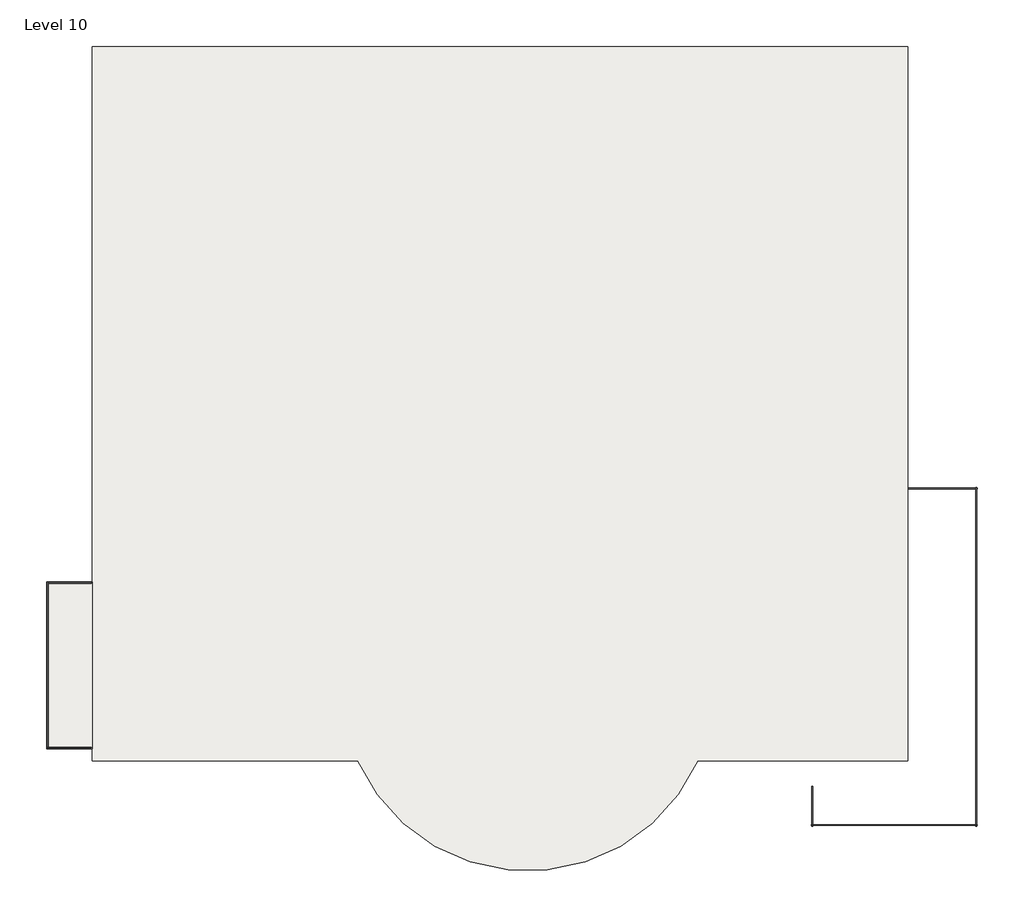
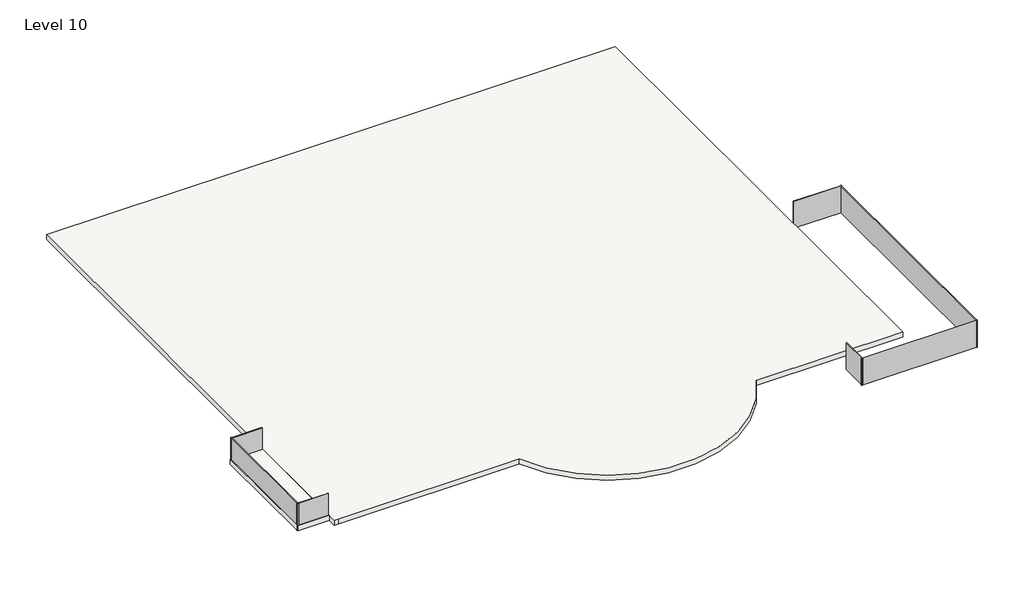
# One storey: 7 plates, 2 slabs.
"""IFC4 building model written with IfcOpenShell, lengths in millimetres."""

from ifc_helpers import new_model, si_unit, point, frame, frame_2d, origin, place, context, project, spatial, polyline, circle_curve, trimmed, segment, composite_curve, outline, extrude, transform, mapped, element, save
from components import system_panel_glazed_7d767388, system_panel_glazed_a5f349e9, system_panel_glazed_524a14c5, system_panel_glazed_4fcd3a06, system_panel_glazed_f6fb2dd6, system_panel_glazed_9d7bd240

model = new_model("IFC4")

# Units and contexts
model_context = context("Model", 3, world=origin())
ifc_project = project(units=[si_unit("LENGTHUNIT", "METRE", prefix="MILLI")], contexts=[model_context])

# Site, building, storey
site = spatial("IfcSite", under=ifc_project)
building = spatial("IfcBuilding", under=site)
storey = spatial("IfcBuildingStorey", under=building, Name="Level 10", Elevation=16154.4)

# Plates
placement = place(None, origin())
system_panel_glazed_shape = system_panel_glazed_7d767388(model_context)
element("IfcPlate", 1, ObjectType="System Panel : Glazed", at=placement, inside=storey, context=model_context, shape_type="MappedRepresentation", body=[
    mapped(system_panel_glazed_shape, transform((-17306.4505427, -8690.0239591, 16154.4), x_axis=(-1.0, 0.0, 0.0), y_axis=(0.0, -1.0, 0.0), z_axis=(0.0, 0.0, 1.0))),
])
element("IfcPlate", 2, ObjectType="System Panel : Glazed", at=placement, inside=storey, context=model_context, shape_type="MappedRepresentation", body=[
    mapped(system_panel_glazed_shape, transform((-17306.4505427, -13712.8739591, 16154.4), x_axis=(1.0, 0.0, 0.0), y_axis=(0.0, 1.0, 0.0), z_axis=(0.0, 0.0, 1.0))),
])
system_panel_glazed_2_shape = system_panel_glazed_a5f349e9(model_context)
element("IfcPlate", 3, ObjectType="System Panel : Glazed", at=placement, inside=storey, context=model_context, shape_type="MappedRepresentation", body=[
    mapped(system_panel_glazed_2_shape, transform((-17979.5505427, -11201.4489591, 16154.4), x_axis=(0.0, -1.0, 0.0), y_axis=(1.0, 0.0, 0.0), z_axis=(0.0, 0.0, 1.0))),
])
system_panel_glazed_3_shape = system_panel_glazed_524a14c5(model_context)
element("IfcPlate", 4, ObjectType="System Panel : Glazed", at=placement, inside=storey, context=model_context, shape_type="MappedRepresentation", body=[
    mapped(system_panel_glazed_3_shape, transform((10079.5464352, -10946.5778294, 16154.4), x_axis=(0.0, 1.0, 0.0), y_axis=(-1.0, 0.0, 0.0), z_axis=(0.0, 0.0, 1.0))),
])
system_panel_glazed_4_shape = system_panel_glazed_4fcd3a06(model_context)
element("IfcPlate", 5, ObjectType="System Panel : Glazed", at=placement, inside=storey, context=model_context, shape_type="MappedRepresentation", body=[
    mapped(system_panel_glazed_4_shape, transform((9038.1464352, -5841.1778294, 16154.4), x_axis=(-1.0, 0.0, 0.0), y_axis=(0.0, -1.0, 0.0), z_axis=(0.0, 0.0, 1.0))),
])
system_panel_glazed_5_shape = system_panel_glazed_f6fb2dd6(model_context)
element("IfcPlate", 6, ObjectType="System Panel : Glazed", at=placement, inside=storey, context=model_context, shape_type="MappedRepresentation", body=[
    mapped(system_panel_glazed_5_shape, transform((5063.0464352, -15455.0778294, 16154.4), x_axis=(0.0, -1.0, 0.0), y_axis=(1.0, 0.0, 0.0), z_axis=(0.0, 0.0, 1.0))),
])
system_panel_glazed_6_shape = system_panel_glazed_9d7bd240(model_context)
element("IfcPlate", 7, ObjectType="System Panel : Glazed", at=placement, inside=storey, context=model_context, shape_type="MappedRepresentation", body=[
    mapped(system_panel_glazed_6_shape, transform((7571.2964352, -16051.9778294, 16154.4), x_axis=(1.0, 0.0, 0.0), y_axis=(0.0, 1.0, 0.0), z_axis=(0.0, 0.0, 1.0))),
])

# Slabs
element("IfcSlab", 8, ObjectType="9\"", at=placement, inside=storey, context=model_context, shape_type="SweptSolid", body=[
    extrude(outline(composite_curve([segment(polyline([(-16607.9505427, 7461.1191779), (7979.2494573, 7461.1191779), (7979.2494573, -14078.0808221), (1652.8739931, -14078.0808221)]), True, "CONTINUOUS"), segment(trimmed(circle_curve(frame_2d((-3476.1505427, -11788.3650223)), 5616.9111737), [point((1652.8739931, -14078.0808221))], [point((-8605.1750786, -14078.0808221))], False, "CARTESIAN"), True, "CONTINUOUS"), segment(polyline([(-8605.1750786, -14078.0808221), (-16404.7505427, -14078.0808221), (-16607.9505427, -14078.0808221), (-16607.9505427, 7461.1191779)]), True, "CONTINUOUS")], self_intersect=False)), frame((0.0, 0.0, 16154.4), z_axis=(0.0, 0.0, 1.0), x_axis=(1.0, 0.0, 0.0)), (0.0, 0.0, 1.0), 228.6),
])
element("IfcSlab", 9, ObjectType="9\"", at=placement, inside=storey, context=model_context, shape_type="SweptSolid", body=[
    extrude(outline(polyline([(-17981.0459551, -8690.0239591), (-16609.4459551, -8690.0239591), (-16609.4459551, -13719.2239591), (-17981.0459551, -13719.2239591), (-17981.0459551, -8690.0239591)])), frame((0.0, 0.0, 16154.4), z_axis=(0.0, 0.0, 1.0), x_axis=(1.0, 0.0, 0.0)), (0.0, 0.0, 1.0), 228.6),
])

save(model, "model.ifc")

# Revit data of these elements
# Type "System Panel : Glazed"
#   Construction Type Id = "GSP4R"
#   Analytic Construction = "1/8 in Pilkington single glazing"
#   Visual Light Transmittance = 0.9
#   Solar Heat Gain Coefficient = 0.86
#   Heat Transfer Coefficient (U) = 1.18115 BTU/(h·ft²·°F)
# Type "9\""
#   Assembly Code = "B1010"
#   Function = 0
#   Layers, outside or top first: 0' - 9" no material (function 1)
# Elements 1, 2, 3, 4, 5, 6, 7 (IfcPlate, "System Panel : Glazed")
#   Phase Created = New Construction
#   Materials on its faces: "Glass"
# Element 8 (IfcSlab, "9\"")
#   built-in parameter 1001955 = 1.5708 (stored number, unit not read)
#   Height Offset From Level = 0' - 9"
#   Phase Created = New Construction
#   Materials on its faces: "Default Floor"
# Element 9 (IfcSlab, "9\"")
#   built-in parameter 1001955 = 3.14159 (stored number, unit not read)
#   Height Offset From Level = 0' - 9"
#   Phase Created = New Construction
#   Materials on its faces: "Default Floor"
# Materials
#   "Glass": class "Glass", colour RGB 0 128 192, transparency 0.75, Description = "Soda Lime Glass", Cost = 0
#   "Default Floor": colour RGB 128 128 128, transparency 0
